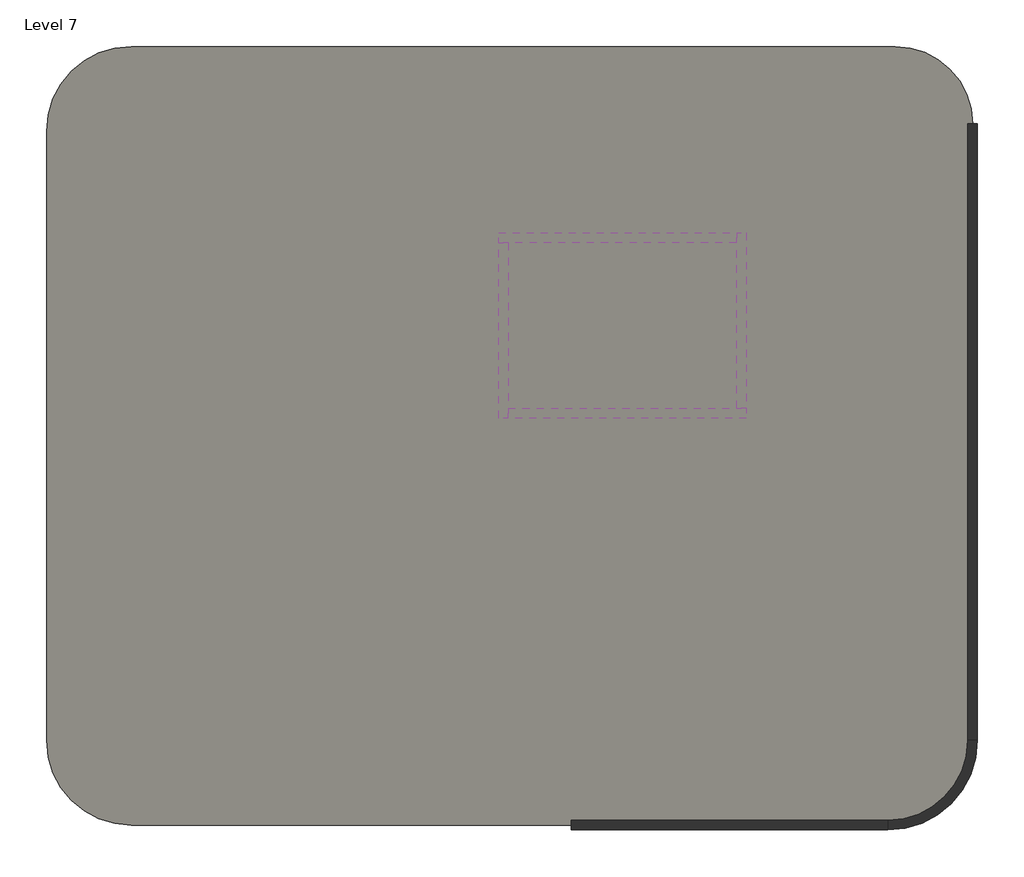
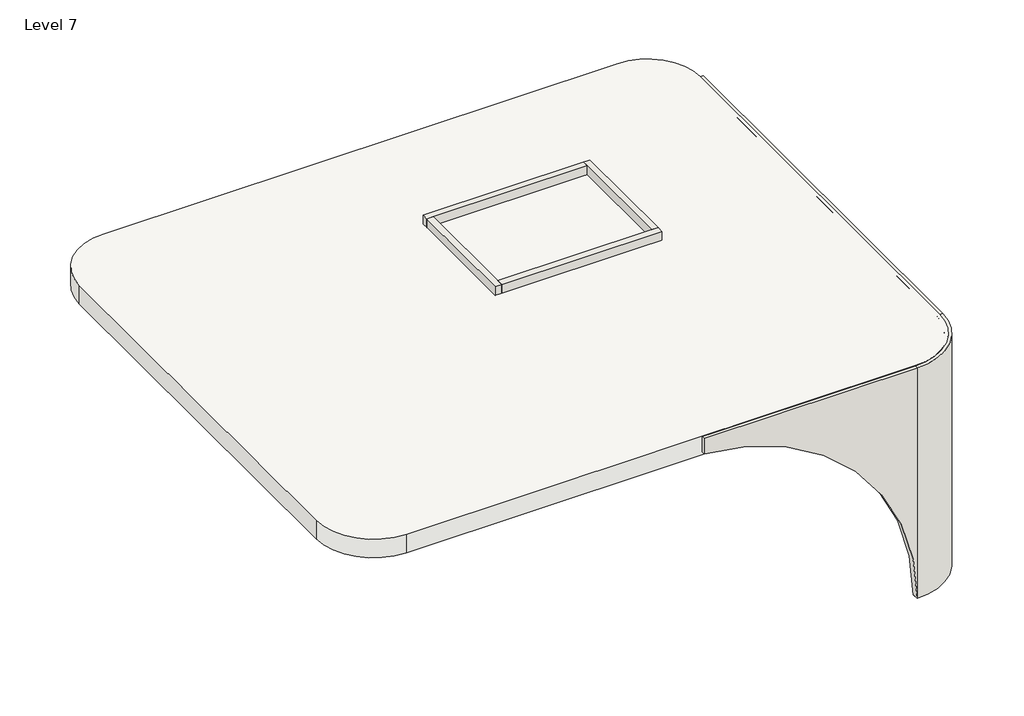
# One storey: 7 walls, 1 slab.
"""IFC4 building model written with IfcOpenShell, lengths in millimetres."""

from ifc_helpers import new_model, si_unit, point, frame, frame_2d, origin, place, context, project, spatial, polyline, circle_curve, trimmed, segment, composite_curve, outline, extrude, faceted_brep, element, save

model = new_model("IFC4")

# Units and contexts
model_context = context("Model", 3, world=origin())
ifc_project = project(units=[si_unit("LENGTHUNIT", "METRE", prefix="MILLI")], contexts=[model_context])

# Site, building, storey
site = spatial("IfcSite", under=ifc_project)
building = spatial("IfcBuilding", under=site)
storey = spatial("IfcBuildingStorey", under=building, Name="Level 7", Elevation=18288.0)

# Slab
placement = place(None, origin())
element("IfcSlab", 1, ObjectType="Generic - 3' white", at=placement, inside=storey, context=model_context, shape_type="SweptSolid", body=[
    extrude(outline(composite_curve([segment(trimmed(circle_curve(frame_2d((1203.8466756, 12828.0432662)), 1625.6), [point((1203.8466756, 14453.6432662))], [point((2829.4466756, 12828.0432662))], False, "CARTESIAN"), True, "CONTINUOUS"), segment(polyline([(2829.4466756, 12828.0432662), (2829.4466756, -125.9567338)]), True, "CONTINUOUS"), segment(trimmed(circle_curve(frame_2d((1051.4466756, -125.9567338)), 1778.0), [point((2829.4466756, -125.9567338))], [point((1051.4466756, -1903.9567338))], False, "CARTESIAN"), True, "CONTINUOUS"), segment(polyline([(1051.4466756, -1903.9567338), (-14848.9533244, -1903.9567338)]), True, "CONTINUOUS"), segment(trimmed(circle_curve(frame_2d((-14848.9533244, -125.9567338)), 1778.0), [point((-14848.9533244, -1903.9567338))], [point((-16626.9533244, -125.9567338))], False, "CARTESIAN"), True, "CONTINUOUS"), segment(polyline([(-16626.9533244, -125.9567338), (-16626.9533244, 12675.6432662)]), True, "CONTINUOUS"), segment(trimmed(circle_curve(frame_2d((-14848.9533244, 12675.6432662)), 1778.0), [point((-16626.9533244, 12675.6432662))], [point((-14848.9533244, 14453.6432662))], False, "CARTESIAN"), True, "CONTINUOUS"), segment(polyline([(-14848.9533244, 14453.6432662), (1203.8466756, 14453.6432662)]), True, "CONTINUOUS")], self_intersect=False)), frame((0.0, 0.0, 18910.3), z_axis=(0.0, 0.0, 1.0), x_axis=(1.0, 0.0, 0.0)), (0.0, 0.0, 1.0), 609.6),
])

# Walls
element("IfcWall", 2, ObjectType="Generic - 8\" white wood", at=placement, inside=storey, context=model_context, shape_type="SweptSolid", body=[
    extrude(outline(composite_curve([segment(trimmed(circle_curve(frame_2d((11893.55, -6072.4903665)), 7123.937042), [point((19002.023072, -5603.3533244))], [point((11893.55, 1051.4466756))], True, "CARTESIAN"), True, "CONTINUOUS"), segment(polyline([(11893.55, 1051.4466756), (19507.2, 1051.4466756), (19507.2, -5603.3533244), (19002.023072, -5603.3533244)]), True, "CONTINUOUS")], self_intersect=False)), frame((0.0, -2005.5567338, 0.0), z_axis=(0.0, 1.0, 0.0), x_axis=(0.0, 0.0, 1.0)), (0.0, 0.0, 1.0), 203.2),
])
element("IfcWall", 3, ObjectType="Generic - 8\" white wood", at=placement, inside=storey, context=model_context, shape_type="SweptSolid", body=[
    extrude(outline(composite_curve([segment(polyline([(2727.8466756, -125.9567338), (2931.0466756, -125.9567338)]), True, "CONTINUOUS"), segment(trimmed(circle_curve(frame_2d((1051.4466756, -125.9567338)), 1879.6), [point((2931.0466756, -125.9567338))], [point((1051.4466756, -2005.5567338))], False, "CARTESIAN"), True, "CONTINUOUS"), segment(polyline([(1051.4466756, -2005.5567338), (1051.4466756, -1802.3567338)]), True, "CONTINUOUS"), segment(trimmed(circle_curve(frame_2d((1051.4466756, -125.9567338)), 1676.4), [point((1051.4466756, -1802.3567338))], [point((2727.8466756, -125.9567338))], True, "CARTESIAN"), True, "CONTINUOUS")], self_intersect=False)), frame((0.0, 0.0, 11893.55), z_axis=(0.0, 0.0, 1.0), x_axis=(1.0, 0.0, 0.0)), (0.0, 0.0, 1.0), 7613.65),
])
element("IfcWall", 4, ObjectType="Generic - 8\" white wood", at=placement, inside=storey, context=model_context, shape_type="SweptSolid", body=[
    extrude(outline(polyline([(2931.0466756, 12828.0432662), (2931.0466756, -125.9567338), (2727.8466756, -125.9567338), (2727.8466756, 12828.0432662), (2931.0466756, 12828.0432662)])), frame((0.0, 0.0, 11893.55), z_axis=(0.0, 0.0, 1.0), x_axis=(1.0, 0.0, 0.0)), (0.0, 0.0, 1.0), 7613.65),
])
element("IfcWall", 5, ObjectType="Generic - 8\" wood", at=placement, inside=storey, context=model_context, shape_type="Brep", body=[
    faceted_brep([(-7131.0978, 10336.3685874, 19507.2), (-6927.8978, 10336.3685874, 19507.2), (-2129.1858906, 10336.3685874, 19507.2), (-2129.1858906, 10336.3685874, 19812.0), (-6927.8978, 10336.3685874, 19812.0), (-7131.0978, 10336.3685874, 19812.0), (-7131.0978, 10539.5685874, 19507.2), (-7131.0978, 10539.5685874, 19812.0), (-2129.1858906, 10539.5685874, 19812.0), (-2129.1858906, 10539.5685874, 19507.2)], [[[0, 1, 2, 3, 4, 5]], [[6, 7, 8, 9]], [[2, 1, 0, 6, 9]], [[5, 4, 3, 8, 7]], [[0, 5, 7, 6]], [[3, 2, 9, 8]]]),
])
element("IfcWall", 6, ObjectType="Generic - 8\" wood", at=placement, inside=storey, context=model_context, shape_type="Brep", body=[
    faceted_brep([(-6927.8978, 6648.0703925, 19507.2), (-6927.8978, 6851.2703925, 19507.2), (-6927.8978, 10336.3685874, 19507.2), (-6927.8978, 10336.3685874, 19812.0), (-6927.8978, 6851.2703925, 19812.0), (-6927.8978, 6648.0703925, 19812.0), (-7131.0978, 6648.0703925, 19507.2), (-7131.0978, 6648.0703925, 19812.0), (-7131.0978, 10336.3685874, 19812.0), (-7131.0978, 10336.3685874, 19507.2)], [[[0, 1, 2, 3, 4, 5]], [[6, 7, 8, 9]], [[2, 1, 0, 6, 9]], [[5, 4, 3, 8, 7]], [[0, 5, 7, 6]], [[3, 2, 9, 8]]]),
])
element("IfcWall", 7, ObjectType="Generic - 8\" wood", at=placement, inside=storey, context=model_context, shape_type="Brep", body=[
    faceted_brep([(-1925.9858906, 6851.2703925, 19507.2), (-2129.1858906, 6851.2703925, 19507.2), (-6927.8978, 6851.2703925, 19507.2), (-6927.8978, 6851.2703925, 19812.0), (-2129.1858906, 6851.2703925, 19812.0), (-1925.9858906, 6851.2703925, 19812.0), (-1925.9858906, 6648.0703925, 19507.2), (-1925.9858906, 6648.0703925, 19812.0), (-6927.8978, 6648.0703925, 19812.0), (-6927.8978, 6648.0703925, 19507.2)], [[[0, 1, 2, 3, 4, 5]], [[6, 7, 8, 9]], [[2, 1, 0, 6, 9]], [[5, 4, 3, 8, 7]], [[0, 5, 7, 6]], [[3, 2, 9, 8]]]),
])
element("IfcWall", 8, ObjectType="Generic - 8\" wood", at=placement, inside=storey, context=model_context, shape_type="Brep", body=[
    faceted_brep([(-2129.1858906, 10539.5685874, 19507.2), (-2129.1858906, 10336.3685874, 19507.2), (-2129.1858906, 6851.2703925, 19507.2), (-2129.1858906, 6851.2703925, 19812.0), (-2129.1858906, 10336.3685874, 19812.0), (-2129.1858906, 10539.5685874, 19812.0), (-1925.9858906, 10539.5685874, 19507.2), (-1925.9858906, 10539.5685874, 19812.0), (-1925.9858906, 6851.2703925, 19812.0), (-1925.9858906, 6851.2703925, 19507.2)], [[[0, 1, 2, 3, 4, 5]], [[6, 7, 8, 9]], [[2, 1, 0, 6, 9]], [[5, 4, 3, 8, 7]], [[0, 5, 7, 6]], [[3, 2, 9, 8]]]),
])

save(model, "model.ifc")

# Revit data of these elements
# Type "Generic - 3' white"
#   Assembly Code = "B1010"
#   Function = 0
#   Layers, outside or top first: 2' - 0" "Tile, Porcelain, 4in" (function 1)
# Type "Generic - 8\" white wood"
#   Assembly Code = "B2010"
#   Layers, outside or top first: 0' - 8" "Tile, Porcelain, 4in" (function 1)
# Type "Generic - 8\" wood"
#   Assembly Code = "B2010"
#   Layers, outside or top first: 0' - 8" "Cherry" (function 1)
# Element 1 (IfcSlab, "Generic - 3' white")
#   Height Offset From Level = 4' - 0 1/2"
#   Phase Created = New Construction
#   Materials on its faces: "Tile, Porcelain, 4in"
# Elements 2, 4 (IfcWall, "Generic - 8\" white wood")
#   built-in parameter 1001111 = -20' - 11 3/4"
#   Top Offset = 0' - 0"
#   Base Offset = -20' - 11 3/4"
#   Unconnected Height = 24' - 11 3/4"
#   wall height = 24' - 11 3/4"
#   Phase Created = New Construction
#   Base Constraint = Level 7
#   Materials on its faces: "Tile, Porcelain, 4in"
# Element 3 (IfcWall, "Generic - 8\" white wood")
#   built-in parameter 1001111 = -20' - 11 3/4"
#   Top Offset = 0' - 0"
#   Base Offset = -20' - 11 3/4"
#   Unconnected Height = 24' - 11 3/4"
#   wall height = 24' - 11 3/4"
#   Phase Created = New Construction
#   Materials on its faces: "Tile, Porcelain, 4in"
# Elements 5, 6, 7, 8 (IfcWall, "Generic - 8\" wood")
#   built-in parameter 1001111 = 4' - 0"
#   Top Offset = 0' - 0"
#   Base Offset = 4' - 0"
#   Unconnected Height = 1' - 0"
#   wall height = 1' - 0"
#   Phase Created = New Construction
#   Base Constraint = Level 7
#   Materials on its faces: "Cherry"
# Materials
#   "Tile, Porcelain, 4in": class "Generic", colour RGB 89 87 158, transparency 0, Description = "Porcelain tile, 4\", white", Cost = 0
#   "Cherry": class "Wood", colour RGB 238 208 179, transparency 0, Description = "Prunus Serotina", Cost = 0
